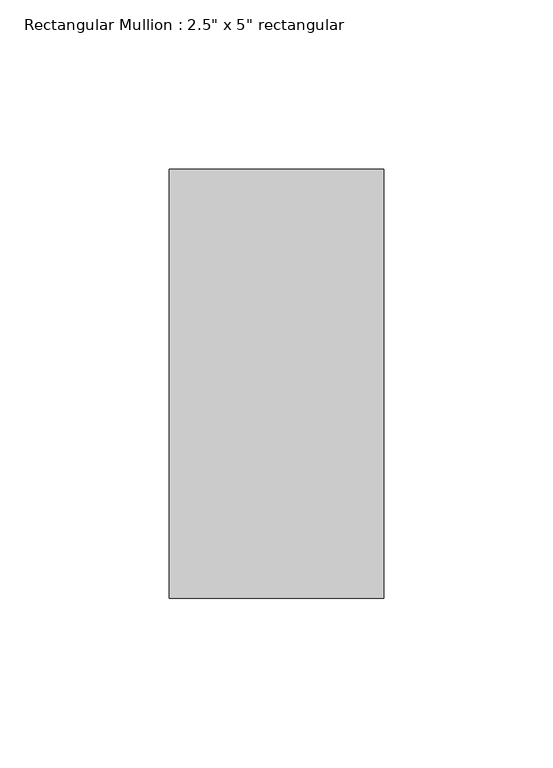
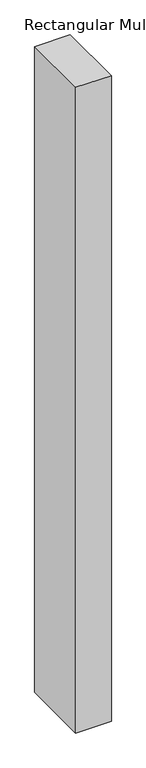
"""IFC4 building model written with IfcOpenShell, lengths in millimetres: member geometry."""

from ifc_helpers import new_model, si_unit, frame, origin, place, context, project, spatial, polyline, outline, extrude, source, transform, mapped, element, save


def member_75074519(model_context):
    return source(origin(), model_context, "Body", "SweptSolid", [
        extrude(outline(polyline([(0.0, 63.5), (0.0, -63.5), (-63.5, -63.5), (-63.5, 63.5), (0.0, 63.5)])), frame((0.0, 0.0, -1219.2), z_axis=(0.0, 0.0, 1.0), x_axis=(1.0, 0.0, 0.0)), (0.0, 0.0, 1.0), 1219.2),
    ])


if __name__ == "__main__":
    model = new_model("IFC4")
    model_context = context("Model", 3, world=origin())
    ifc_project = project(units=[si_unit("LENGTHUNIT", "METRE", prefix="MILLI")], contexts=[model_context])
    site = spatial("IfcSite", under=ifc_project)
    building = spatial("IfcBuilding", under=site)
    placement = place(None, origin())
    member_shape = member_75074519(model_context)
    element("IfcMember", 1, ObjectType="Rectangular Mullion : 2.5\" x 5\" rectangular", at=placement, inside=building, context=model_context, shape_type="MappedRepresentation", body=[
        mapped(member_shape, transform((0.0, 0.0, 0.0), x_axis=(1.0, 0.0, 0.0), y_axis=(0.0, 1.0, 0.0), z_axis=(0.0, 0.0, 1.0))),
    ])
    save(model, "model.ifc")

# Revit data of these elements
# Type "Rectangular Mullion : 2.5\" x 5\" rectangular"
#   built-in parameter 1007304 = 0.416667 (stored number, unit not read)
#   built-in parameter 1007301 = 0.104167 (stored number, unit not read)
#   built-in parameter 1007300 = 0.104167 (stored number, unit not read)
# Element 1 (IfcMember, "Rectangular Mullion : 2.5\" x 5\" rectangular")
#   Materials on its faces: "Aluminum"
# Materials
#   "Aluminum": class "Metal", colour RGB 247 247 247, transparency 0, Description = "Aluminum 6061", Cost = 0
